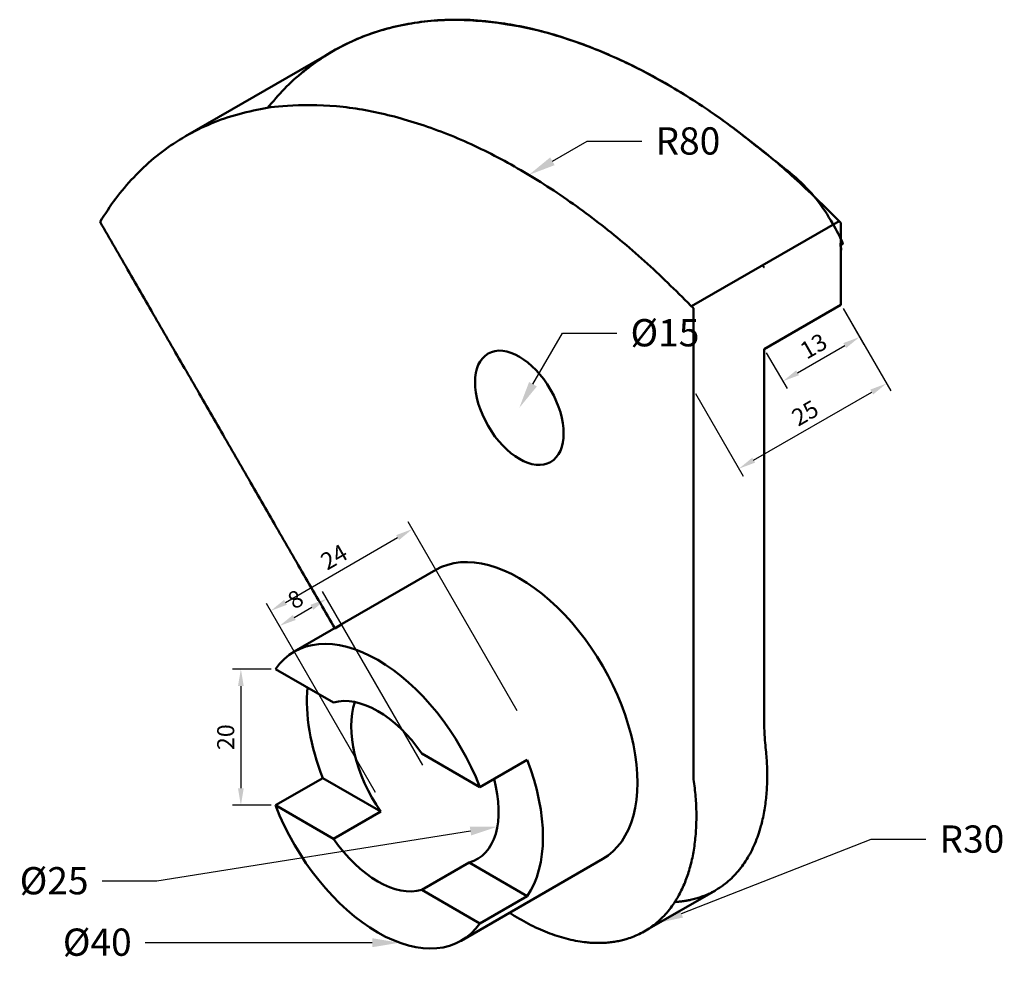
# Model space of a CAD drawing. Units: millimetres. Extents: x 2925 to 3069, y 1736 to 1874.
import ezdxf
from ezdxf import colors
from ezdxf.entities.mleader import LeaderData, LeaderLine
from ezdxf.math import Vec2, Vec3

# ---------------------------------------------------------------- set-up
doc = ezdxf.new("R2010")
doc.units = ezdxf.units.MM
doc.layers.add('M-DIMS', color=2, linetype='Continuous', lineweight=25)
doc.layers.add('M-OUTL', color=7, linetype='Continuous', lineweight=50)
doc.styles.get("Standard").update_dxf_attribs({"font": 'arial.ttf'})
doc.dimstyles.new('ISO-25', dxfattribs={"dimtxt": 2.5, "dimasz": 2.5, "dimexe": 1.25, "dimexo": 0.625, "dimtad": 1, "dimtxsty": 'Standard', "dimcen": 2.5, "dimadec": 0, "dimazin": 0, "dimtfac": 1, "dimtmove": 0, "dimatfit": 3, "dimfxl": 1, "dimarcsym": 0})

# ---------------------------------------------------------------- blocks, each defined once
blk = doc.blocks.new('*D1')
at = {"layer": 'Defpoints', "color": 0, "transparency": 16777216}
for p in [(2969.6, 1789.38), (2984.02, 1764.4), (2977.09, 1760.4)]:
    blk.add_point(p, dxfattribs=at)
at = {"layer": 'M-DIMS', "color": 0, "lineweight": -2, "transparency": 16777216}
for p, q in [((2983.71, 1764.94), (2968.98, 1790.46)), ((2964.84, 1786.63), (2967.44, 1788.13)), ((2976.78, 1760.94), (2962.05, 1786.46))]:
    blk.add_line(p, q, dxfattribs=at)
at = {"layer": 'M-DIMS', "color": 0, "transparency": 16777216}
for points in [[(2967.23, 1788.49), (2967.64, 1787.76), (2969.6, 1789.38)], [(2964.63, 1786.99), (2965.05, 1786.26), (2962.67, 1785.38)]]:
    blk.add_solid(points, dxfattribs=at)
at = {"layer": 'M-DIMS', "color": 0, "transparency": 16777216, "insert": (2965.19, 1789.02), "char_height": 2.5, "attachment_point": 5, "rotation": 30}
blk.add_mtext('8', dxfattribs=at)
blk = doc.blocks.new('*D2')
at = {"layer": 'Defpoints', "color": 0, "transparency": 16777216}
for p in [(2982.17, 1799.6), (2997.88, 1772.4), (2977.09, 1760.4)]:
    blk.add_point(p, dxfattribs=at)
at = {"layer": 'M-DIMS', "color": 0, "lineweight": -2, "transparency": 16777216}
for p, q in [((2997.56, 1772.94), (2981.55, 1800.68)), ((2963.55, 1788.85), (2980.01, 1798.35)), ((2976.78, 1760.94), (2960.76, 1788.68))]:
    blk.add_line(p, q, dxfattribs=at)
at = {"layer": 'M-DIMS', "color": 0, "transparency": 16777216}
for points in [[(2979.8, 1798.71), (2980.22, 1797.99), (2982.17, 1799.6)], [(2963.35, 1789.21), (2963.76, 1788.49), (2961.39, 1787.6)]]:
    blk.add_solid(points, dxfattribs=at)
at = {"layer": 'M-DIMS', "color": 0, "transparency": 16777216, "insert": (2970.84, 1795.23), "char_height": 2.5, "attachment_point": 5, "rotation": 30}
blk.add_mtext('24', dxfattribs=at)
blk = doc.blocks.new('*D3')
at = {"layer": 'Defpoints', "color": 0, "transparency": 16777216}
for p in [(2962.09, 1779.06), (2957.01, 1759.06), (2962.09, 1759.06)]:
    blk.add_point(p, dxfattribs=at)
at = {"layer": 'M-DIMS', "color": 0, "lineweight": -2, "transparency": 16777216}
for p, q in [((2961.47, 1779.06), (2955.76, 1779.06)), ((2957.01, 1776.56), (2957.01, 1761.56)), ((2961.47, 1759.06), (2955.76, 1759.06))]:
    blk.add_line(p, q, dxfattribs=at)
at = {"layer": 'M-DIMS', "color": 0, "transparency": 16777216}
for points in [[(2956.59, 1776.56), (2957.43, 1776.56), (2957.01, 1779.06)], [(2956.59, 1761.56), (2957.43, 1761.56), (2957.01, 1759.06)]]:
    blk.add_solid(points, dxfattribs=at)
at = {"layer": 'M-DIMS', "color": 0, "transparency": 16777216, "insert": (2955.11, 1769.06), "char_height": 2.5, "attachment_point": 5, "rotation": 90}
blk.add_mtext('20', dxfattribs=at)
blk = doc.blocks.new('*D4')
at = {"layer": 'Defpoints', "color": 0, "transparency": 16777216}
for p in [(3045.07, 1832.52), (3047.8, 1827.79), (3033.81, 1826.02)]:
    blk.add_point(p, dxfattribs=at)
at = {"layer": 'M-DIMS', "color": 0, "lineweight": -2, "transparency": 16777216}
for p, q in [((3045.38, 1831.98), (3048.42, 1826.71)), ((3038.71, 1822.54), (3045.63, 1826.54)), ((3034.12, 1825.48), (3037.17, 1820.21))]:
    blk.add_line(p, q, dxfattribs=at)
at = {"layer": 'M-DIMS', "color": 0, "transparency": 16777216}
for points in [[(3045.43, 1826.9), (3045.84, 1826.18), (3047.8, 1827.79)], [(3038.5, 1822.9), (3038.91, 1822.18), (3036.54, 1821.29)]]:
    blk.add_solid(points, dxfattribs=at)
at = {"layer": 'M-DIMS', "color": 0, "transparency": 16777216, "insert": (3041.22, 1826.19), "char_height": 2.5, "attachment_point": 5, "rotation": 30}
blk.add_mtext('13', dxfattribs=at)
blk = doc.blocks.new('*D5')
at = {"layer": 'Defpoints', "color": 0, "transparency": 16777216}
for p in [(3045.07, 1832.52), (3051.74, 1820.96), (3023.42, 1820.02)]:
    blk.add_point(p, dxfattribs=at)
at = {"layer": 'M-DIMS', "color": 0, "lineweight": -2, "transparency": 16777216}
for p, q in [((3045.38, 1831.98), (3052.37, 1819.87)), ((3023.73, 1819.48), (3030.72, 1807.37)), ((3032.26, 1809.71), (3049.58, 1819.71))]:
    blk.add_line(p, q, dxfattribs=at)
at = {"layer": 'M-DIMS', "color": 0, "transparency": 16777216}
for points in [[(3049.37, 1820.07), (3049.79, 1819.35), (3051.74, 1820.96)], [(3032.05, 1810.07), (3032.47, 1809.35), (3030.09, 1808.46)]]:
    blk.add_solid(points, dxfattribs=at)
at = {"layer": 'M-DIMS', "color": 0, "transparency": 16777216, "insert": (3039.97, 1816.35), "char_height": 2.5, "attachment_point": 5, "rotation": 30}
blk.add_mtext('25', dxfattribs=at)

msp = doc.modelspace()

# ---------------------------------------------------------------- linework, layer by layer
at = {"layer": 'M-OUTL'}
for p, q in [((2970.538, 1869.753), (2948.887, 1857.253)), ((3023.135, 1832.312), (3044.786, 1844.812)), ((3045.066, 1844.523), (3045.066, 1832.523)), ((3045.066, 1832.523), (3033.807, 1826.023)), ((2964.845, 1781.614), (2985.63, 1793.614)), ((2970.597, 1774.15), (2962.093, 1779.061)), ((2983.588, 1766.65), (2992.093, 1761.74)), ((2992.093, 1761.74), (2999.021, 1765.74)), ((2962.093, 1759.061), (2969.021, 1763.061)), ((2977.526, 1758.15), (2969.021, 1763.061)), ((2970.597, 1754.15), (2962.093, 1759.061)), ((2970.597, 1754.15), (2977.526, 1758.15)), ((2983.588, 1746.65), (2990.516, 1750.65)), ((2989.34, 1739.187), (3010.125, 1751.187)), ((2990.516, 1750.65), (2999.021, 1745.74)), ((2983.588, 1746.65), (2992.093, 1741.74)), ((2992.093, 1741.74), (2999.021, 1745.74)), ((3026.641, 1746.581), (3016.249, 1740.581))]:
    msp.add_line(p, q, dxfattribs=at)
msp.add_ellipse((2997.877, 1817.4), major_axis=(4.593, -7.955), ratio=0.5773503, dxfattribs=at)
for centre, major_axis, start_param, end_param in [((2997.877, 1772.4), (12.247, -21.213), 6.2831853, 9.424778), ((2984.021, 1764.4), (12.247, -21.213), 9.424778, 9.5054144), ((2977.093, 1760.4), (12.247, -21.213), 7.5921822, 9.6865773), ((2984.021, 1764.4), (12.247, -21.213), 10.1100087, 10.7337749), ((2977.093, 1760.4), (7.655, -13.258), 7.9958787, 9.2828809), ((2984.021, 1764.4), (7.655, -13.258), 3.6112136, 4.854286), ((2984.021, 1764.4), (12.247, -21.213), 6.5449847, 7.5921822), ((2984.021, 1764.4), (7.655, -13.258), 6.1412883, 7.4270163), ((2977.093, 1760.4), (12.247, -21.213), 4.4505896, 6.5449847), ((2977.093, 1760.4), (7.655, -13.258), 4.854286, 6.1412883), ((2984.021, 1764.4), (12.247, -21.213), 6.2831853, 6.2964439)]:
    msp.add_ellipse(centre, major_axis=major_axis, ratio=0.5773503, start_param=start_param, end_param=end_param, dxfattribs=at)
for points, weights in [([(3045.066, 1844.523), (2991.601, 1899.871), (2960.924, 1861.406)], [1, 0.757705092462, 0.969774056281]), ([(3023.415, 1832.023), (2965.154, 1892.336), (2936.347, 1844.695)], [1, 0.741586750533, 1]), ([(3033.807, 1838.023), (3033.668, 1838.168), (3033.528, 1838.312)], [1, 0.999164394947, 0.998334193919])]:
    msp.add_rational_spline(points, weights, degree=2, dxfattribs=at)
for points, weights, knots in [([(3045.066, 1832.523), (3045.066, 1838.523), (3045.066, 1844.523), (2997.211, 1894.063), (2965.233, 1865.941)], [1, 1, 1, 0.777472224412, 0.938195779863], [4.9969404, 4.9969404, 4.9969404, 5.1712287, 5.1712287, 6.4377185, 6.4377185, 6.4377185]), ([(3020.694, 1744.88), (3022.983, 1744.998), (3024.979, 1745.781), (3036.597, 1750.341), (3033.807, 1769.171), (3033.807, 1797.597), (3033.807, 1826.023)], [0.957379065681, 0.973570479124, 1, 0.863545176037, 1, 1, 1], [2.9094106, 2.9094106, 2.9094106, 3.1141525, 3.1141525, 4.1712287, 4.1712287, 4.9969404, 4.9969404, 4.9969404]), ([(2996.43, 1743.283), (3006.706, 1736.688), (3014.587, 1739.781), (3026.204, 1744.341), (3023.415, 1763.171)], [0.943754005975, 0.903181310694, 1, 0.863545176037, 1], [2.364126, 2.364126, 2.364126, 3.1141525, 3.1141525, 4.1712287, 4.1712287, 4.1712287])]:
    msp.add_rational_spline(points, weights, degree=2, knots=knots, dxfattribs=at)
for points in [[(2936.347, 1844.695), (2953.587, 1814.835), (2970.827, 1784.975)], [(3023.415, 1763.171), (3023.415, 1797.597), (3023.415, 1832.023)]]:
    msp.add_open_spline(points, degree=2, dxfattribs=at)

# ---------------------------------------------------------------- dimensions: what is measured, and where the dimension line sits
at = {"layer": 'M-DIMS'}
for p1, p2, distance, picture, middle in [((3023.415, 1820.023), (3045.066, 1832.523), -13.356, '*D5', (3039.968, 1816.353)), ((3033.807, 1826.023), (3045.066, 1832.523), -5.467, '*D4', (3041.219, 1826.186)), ((2977.093, 1760.4), (2997.877, 1772.4), 31.408, '*D2', (2970.841, 1795.228)), ((2977.093, 1760.4), (2984.021, 1764.4), 28.839, '*D1', (2965.186, 1789.022)), ((2962.093, 1779.061), (2962.093, 1759.061), -5.081, '*D3', (2955.11, 1769.061))]:
    dim = msp.add_aligned_dim(p1=p1, p2=p2, distance=distance, dimstyle='ISO-25', override={"dimclrd": 0, "dimclre": 0, "dimclrt": 0}, dxfattribs=at)
    dim.commit()
    dim.dimension.update_dxf_attribs({"geometry": picture, "text_midpoint": middle})

# ---------------------------------------------------------------- leaders
ml = msp.add_multileader_mtext('Standard', dxfattribs=at)
ml.set_content('R80', color=256)
ml.set_leader_properties()
ml.build(insert=Vec2(0, 0))
ctx = ml.context
ctx.base_point, ctx.plane_origin = Vec3(3015.847, 1856.533), Vec3(2999.269, 1851.58)
notes = []
notes.append((ctx, [(0, (1, 1, 0), (3007.847, 1856.533), (1, 0), 8, [(0, [(2999.269, 1851.58)], 0, [])])]))
ctx.mtext.insert, ctx.mtext.flow_direction = Vec3(3017.847, 1858.567), 5
ml = msp.add_multileader_mtext('Standard', dxfattribs=at)
ml.set_content('%%C15', color=256)
ml.set_leader_properties()
ml.build(insert=Vec2(0, 0))
ctx = ml.context
ctx.base_point, ctx.plane_origin = Vec3(3012.19, 1828.334), Vec3(2997.877, 1817.4)
notes.append((ctx, [(0, (1, 1, 0), (3004.19, 1828.334), (1, 0), 8, [(0, [(2997.877, 1817.4)], 0, [])])]))
ctx.mtext.insert, ctx.mtext.flow_direction = Vec3(3014.19, 1830.415), 5
ml = msp.add_multileader_mtext('Standard', dxfattribs=at)
ml.set_content('%%C25', color=256)
ml.set_leader_properties()
ml.build(insert=Vec2(0, 0))
ctx = ml.context
ctx.base_point, ctx.plane_origin = Vec3(2922.548, 1747.913), Vec3(2994.656, 1755.925)
ctx.text_align_type = 2
notes.append((ctx, [(0, (1, 1, 0), (2944.659, 1747.913), (-1, 0), 8, [(0, [(2994.656, 1755.925)], 0, [])])]))
ctx.mtext.insert, ctx.mtext.alignment, ctx.mtext.flow_direction = Vec3(2934.659, 1749.994), 3, 5
ml = msp.add_multileader_mtext('Standard', dxfattribs=at)
ml.set_content('R30', color=256)
ml.set_leader_properties()
ml.build(insert=Vec2(0, 0))
ctx = ml.context
ctx.base_point, ctx.plane_origin = Vec3(3057.522, 1754.074), Vec3(3017.929, 1741.748)
notes.append((ctx, [(0, (1, 1, 0), (3049.522, 1754.074), (1, 0), 8, [(0, [(3017.929, 1741.748)], 0, [])])]))
ctx.mtext.insert, ctx.mtext.flow_direction = Vec3(3059.522, 1756.11), 5
ml = msp.add_multileader_mtext('Standard', dxfattribs=at)
ml.set_content('%%C40', color=256)
ml.set_leader_properties()
ml.build(insert=Vec2(0, 0))
ctx = ml.context
ctx.base_point, ctx.plane_origin = Vec3(2928.921, 1738.897), Vec3(2980.292, 1738.897)
ctx.text_align_type = 2
notes.append((ctx, [(0, (1, 1, 0), (2950.99, 1738.897), (-1, 0), 8, [(0, [(2980.292, 1738.897)], 0, [])])]))
ctx.mtext.insert, ctx.mtext.alignment, ctx.mtext.flow_direction = Vec3(2940.99, 1740.978), 3, 5
for ctx, leaders in notes:
    for number, flags, end, landing, length, lines in leaders:
        leader = LeaderData()
        leader.index, (leader.has_last_leader_line, leader.has_dogleg_vector, leader.attachment_direction) = number, flags
        leader.last_leader_point, leader.dogleg_vector, leader.dogleg_length = Vec3(end), Vec3(landing), length
        for number, points, colour, breaks in lines:
            line = LeaderLine()
            line.index, line.vertices, line.color, line.breaks = number, Vec3.list(points), colors.encode_raw_color(colour), breaks
            leader.lines.append(line)
        ctx.leaders.append(leader)

doc.saveas('drawing.dxf')
